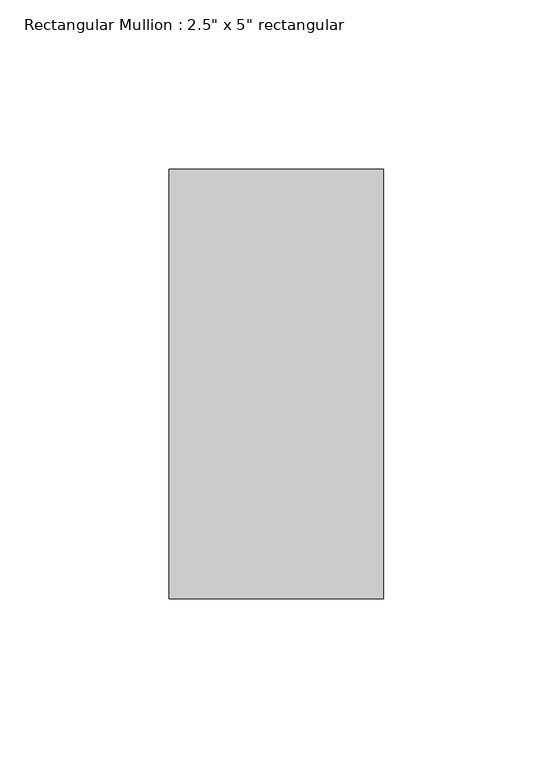
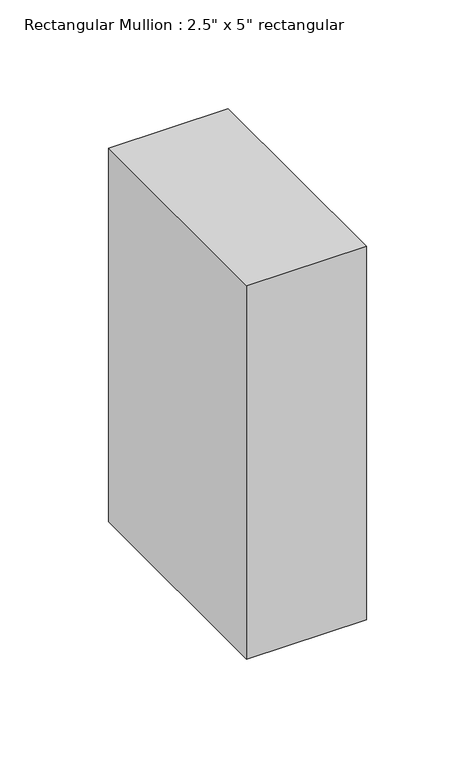
"""IFC4 building model written with IfcOpenShell, lengths in millimetres: member geometry."""

from ifc_helpers import new_model, si_unit, frame, origin, place, context, project, spatial, polyline, outline, extrude, source, transform, mapped, element, save


def member_420b45ef(model_context):
    return source(origin(), model_context, "Body", "SweptSolid", [
        extrude(outline(polyline([(0.0, 63.5), (0.0, -63.5), (-63.5, -63.5), (-63.5, 63.5), (0.0, 63.5)])), frame((0.0, 0.0, -209.55), z_axis=(0.0, 0.0, 1.0), x_axis=(1.0, 0.0, 0.0)), (0.0, 0.0, 1.0), 209.55),
    ])


if __name__ == "__main__":
    model = new_model("IFC4")
    model_context = context("Model", 3, world=origin())
    ifc_project = project(units=[si_unit("LENGTHUNIT", "METRE", prefix="MILLI")], contexts=[model_context])
    site = spatial("IfcSite", under=ifc_project)
    building = spatial("IfcBuilding", under=site)
    placement = place(None, origin())
    member_shape = member_420b45ef(model_context)
    element("IfcMember", 1, ObjectType="Rectangular Mullion : 2.5\" x 5\" rectangular", at=placement, inside=building, context=model_context, shape_type="MappedRepresentation", body=[
        mapped(member_shape, transform((0.0, 0.0, 0.0), x_axis=(1.0, 0.0, 0.0), y_axis=(0.0, 1.0, 0.0), z_axis=(0.0, 0.0, 1.0))),
    ])
    save(model, "model.ifc")

# Revit data of these elements
# Type "Rectangular Mullion : 2.5\" x 5\" rectangular"
#   built-in parameter 1007304 = 0.416667 (stored number, unit not read)
#   built-in parameter 1007301 = 0.104167 (stored number, unit not read)
#   built-in parameter 1007300 = 0.104167 (stored number, unit not read)
# Element 1 (IfcMember, "Rectangular Mullion : 2.5\" x 5\" rectangular")
#   Materials on its faces: "Aluminum"
# Materials
#   "Aluminum": class "Metal", colour RGB 247 247 247, transparency 0, Description = "Aluminum 6061", Cost = 0
